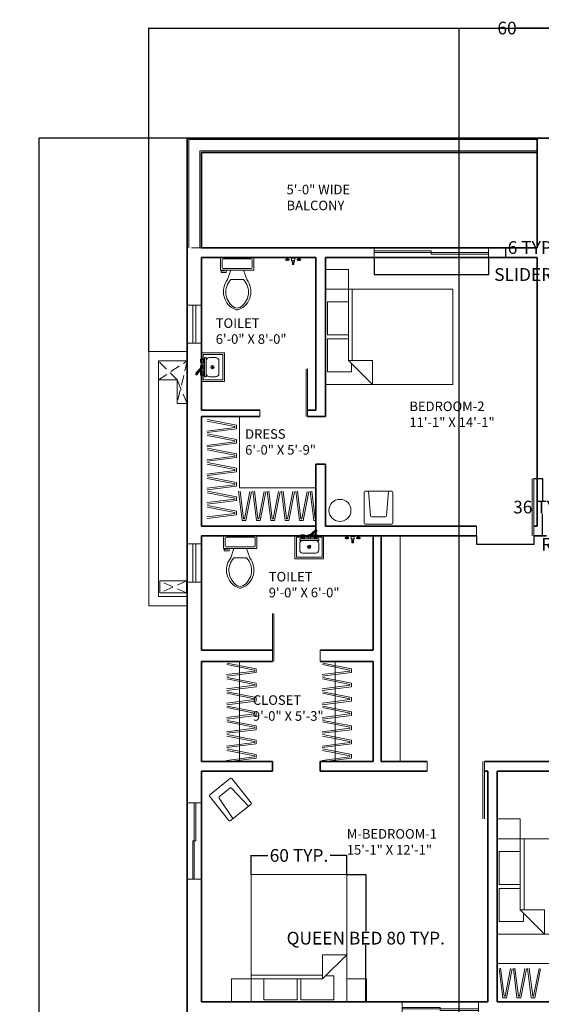
# Model space of a CAD drawing. Units: inches. Extents: x 3343 to 4790, y 1140 to 2641.
# Tile 3 of 10: x 3343 to 3671, y 2022 to 2641. Entities that reach past the tile are written whole.
import ezdxf

# ---------------------------------------------------------------- set-up
doc = ezdxf.new("R2010")
doc.units = ezdxf.units.IN
doc.header["$LTSCALE"] = 5
doc.header["$MEASUREMENT"] = 0
doc.linetypes.add('HIDDEN', pattern=[0.375, 0.25, -0.125])
for name, color, linetype, lineweight in [('A-ANNO-DIMS', 2, 'Continuous', 18), ('A-AREA-IDEN', 7, 'Continuous', 18), ('A-DOOR', 3, 'Continuous', 18), ('A-FLOR-CASE', 9, 'Continuous', 18), ('A-FLOR-FIXT', 9, 'Continuous', 18), ('A-FLOR-HIDN', 8, 'HIDDEN', 13), ('A-FLOR-RAIL', 7, 'Continuous', 18), ('A-FLOR-SHFT', 8, 'Continuous', 18), ('A-FURN', 8, 'Continuous', 13), ('A-GLAZ', 4, 'Continuous', 18), ('A-WALL', 7, 'Continuous', 35)]:
    doc.layers.add(name, color=color, linetype=linetype, lineweight=lineweight)
doc.styles.get("Standard").update_dxf_attribs({"font": 'arial.ttf'})
doc.dimstyles.get("Standard").update_dxf_attribs({"dimtxt": 8, "dimasz": 0.18, "dimexe": 0.18, "dimexo": 0.0625, "dimgap": 0.09, "dimtad": 0, "dimtih": 1, "dimtoh": 1, "dimdec": 1, "dimzin": 0, "dimdsep": 46, "dimlunit": 3, "dimtxsty": 'Standard', "dimcen": 0.09, "dimadec": 0, "dimazin": 0, "dimtfac": 1, "dimtdec": 1, "dimtofl": 0, "dimtmove": 0, "dimatfit": 3, "dimfxl": 1, "dimtolj": 1, "dimtzin": 0, "dimarcsym": 0})

# ---------------------------------------------------------------- blocks, each defined once
blk = doc.blocks.new('Bed - Queen')
for p, q in [((0, -80.00003), (0, 0)), ((0, 0), (59.99999, 0)), ((59.99999, 0), (59.99999, -80.00003)), ((7.99999, -1.2), (28.79998, -1.2)), ((7.99999, -14.4), (7.99999, -1.2)), ((28.79998, -1.2), (28.79998, -14.4)), ((31.19999, -1.2), (51.99999, -1.2)), ((31.19999, -14.4), (31.19999, -1.2)), ((51.99999, -1.2), (51.99999, -16.4)), ((0, -14.4), (44.8, -14.4)), ((44.8, -16.8), (0, -16.8)), ((59.99999, -29.6), (44.8, -14.4)), ((44.8, -14.4), (44.8, -29.6)), ((51.99999, -16.4), (46.79936, -16.4)), ((44.8, -29.6), (59.99999, -29.6)), ((59.99999, -80.00003), (0, -80.00003))]:
    blk.add_line(p, q)
blk = doc.blocks.new('Toilet - top')
for p, q in [((9.5, -6), (9.5, -2)), ((-10, -8.5), (-8, -8.5)), ((-10, -9.5), (-10, -8.5)), ((-7, -9.5), (-10, -9.5)), ((-8, -8.5), (-8, -8)), ((-7, -8), (-7, -9.5)), ((-4, -8), (-6, -14)), ((4, -8), (6, -14)), ((4, -14), (-4, -14))]:
    blk.add_line(p, q)
blk.add_lwpolyline([(10.5, -8), (10.5, 0), (-10.5, 0), (-10.5, -8)], close=True)
for points in [[(-9.5, -2), (-9.5, -6)], [(8.5, -1), (-8.5, -1)], [(-8.5, -7), (8.5, -7)]]:
    blk.add_lwpolyline(points)
for centre, radius, start, end in [((-8.62, -1.88), 0.884, 81.8699, 188.1301), ((-8.62, -6.12), 0.884, 171.8699, 278.1301), ((8.62, -1.88), 0.884, 351.8699, 98.1301), ((8.62, -6.12), 0.884, 261.8699, 8.1301), ((3.52, -21.58), 12.17, 141.46911, 247.97143), ((4.2, -21.82), 11.33, 136.36773, 238.94682), ((-3.52, -21.58), 12.17, 292.02843, 38.53071), ((-4.2, -21.82), 11.33, 301.05301, 43.63209), ((0, -27.88), 4, 245.73182, 294.26817), ((0, -29), 4, 254.86053, 285.13947)]:
    blk.add_arc(centre, radius, start, end)
blk = doc.blocks.new('Faucet - kit sink front')
for p, q in [((-0.25, 3), (3.75, 6.5)), ((3.75, 6), (3.75, 6.5)), ((3.75, 6.5), (4.75, 6.5)), ((4.75, 6.5), (4.75, 6)), ((-4.5, 1), (-4.5, 1.5)), ((-3.5, 1.5), (-3.5, 1)), ((-0.75, 3.5), (0.3192, 3.5)), ((-0.75, 1), (-0.75, 3.5)), ((3.75, 6), (-0.25, 2.5)), ((-0.25, 2.5), (-0.25, 3)), ((0.75, 2.5), (-0.25, 2.5)), ((4.1921, 5.5041), (0.75, 2.5)), ((0.75, 2.5), (0.75, 1)), ((3.5, 1.5), (3.5, 1)), ((3.75, 5.5), (3.75, 6)), ((4.75, 6), (3.75, 6)), ((4.75, 5.5), (3.75, 5.5)), ((4.5, 1), (4.5, 1.5)), ((4.75, 6), (4.75, 5.5))]:
    blk.add_line(p, q)
for points in [[(-6, 0), (-6, 1), (6, 1), (6, 0)], [(-5.5, 2.5), (-5.5, 3.25), (-4.5, 3.25), (-4.5, 2.5)], [(5.5, 2.5), (5.5, 3.25), (4.5, 3.25), (4.5, 2.5)]]:
    blk.add_lwpolyline(points, close=True)
for points in [[(-5, 3.2513), (-5, 3.5), (-3, 3.5), (-3, 1.5), (-5, 1.5), (-5, 2.5)], [(5, 3.2513), (5, 3.5), (3, 3.5), (3, 1.5), (5, 1.5), (5, 2.5)]]:
    blk.add_lwpolyline(points)
blk = doc.blocks.new('Faucet - Bathroom front')
for p, q in [((-5, 0), (-2.25, 0)), ((-4.5087, 0.25), (-2.7408, 0.25)), ((-4, 1.625), (-4.25, 1.625)), ((-4, 1.375), (-4.25, 1.375)), ((-3.1442, 0.75), (-4.0979, 0.75)), ((-3.25, 1.625), (-3, 1.625)), ((-3.25, 1.375), (-3, 1.375)), ((-1.5, 0), (1.5, 0)), ((-1, 0.5), (1, 0.5)), ((-0.5, 4.25), (0.5, 4.25)), ((0.5, 3.75), (-0.5, 3.75)), ((-0.5, 3), (0.5, 3)), ((0.5, 2), (-0.5, 2)), ((-0.25, 3), (-0.25, 3.5)), ((0.25, 3.5), (0.25, 3)), ((2.25, 0), (5, 0)), ((2.7413, 0.25), (4.5092, 0.25)), ((3.25, 1.625), (3, 1.625)), ((3.25, 1.375), (3, 1.375)), ((4.1058, 0.75), (3.1521, 0.75)), ((4, 1.625), (4.25, 1.625)), ((4, 1.375), (4.25, 1.375))]:
    blk.add_line(p, q)
for points in [[(-4, 1), (-4, 2), (-3.25, 2), (-3.25, 1)], [(3.25, 1), (3.25, 2), (4, 2), (4, 1)]]:
    blk.add_lwpolyline(points, close=True)
for points in [[(-0.5, 3.75), (-0.5, 4.25)], [(-0.25, 4.5), (0.25, 4.5)], [(0.25, 3.5), (-0.25, 3.5)], [(0.5, 4.25), (0.5, 3.75)]]:
    blk.add_lwpolyline(points)
for centre in [(-4.5, 1.5), (-3.625, 1.5), (-2.75, 1.5), (2.75, 1.5), (3.625, 1.5), (4.5, 1.5)]:
    blk.add_circle(centre, 0.2795)
for centre, radius, start, end in [((-5.375, 1.375), 1.4252, 285.2551, 344.7449), ((-1.875, 1.375), 1.4252, 195.2551, 254.7449), ((-0.7962, -0.2038), 0.7327, 106.1502, 163.8498), ((3, 1), 4.0311, 150.2551, 187.125), ((0.6413, 2.5), 1.246, 156.3417, 203.6583), ((-0.2575, 4.2575), 0.2426, 88.22243, 181.7776), ((-0.2575, 3.7425), 0.2426, 178.2224, 271.7776), ((0.2575, 4.2575), 0.2426, 358.2224, 91.77757), ((0.2575, 3.7425), 0.2426, 268.2224, 1.777565), ((-3, 1), 4.0311, 352.875, 29.74488), ((-0.6413, 2.5), 1.246, 336.3417, 23.65835), ((0.7962, -0.2038), 0.7327, 16.1502, 73.84979), ((1.875, 1.375), 1.4252, 285.2551, 344.7449), ((5.375, 1.375), 1.4252, 195.2551, 254.7449)]:
    blk.add_arc(centre, radius, start, end)
blk = doc.blocks.new('CHAIR-SIDE')
for p, q in [((0, 0.6), (0, 20.1)), ((0.6, 20.7), (17.39, 20.7)), ((2.68, 20.7), (3.95, 5.17)), ((15.31, 20.7), (14.03, 5.17)), ((17.98, 20.1), (17.98, 0.6)), ((17.39, 0), (0.6, 0)), ((13.44, 4.62), (4.54, 4.62))]:
    blk.add_line(p, q)
for centre, start, end in [((0.6, 20.1), 90, 180), ((17.39, 20.1), 0, 90), ((0.6, 0.6), 180, 270), ((4.54, 5.22), 184.67931, 270), ((13.44, 5.22), 270, 355.32069), ((17.39, 0.6), 270, 0)]:
    blk.add_arc(centre, 0.595, start, end)
blk = doc.blocks.new('SINK-BOWL-WITH-DRAIN')
for p, q in [((8.58, 9.03), (6.47, 9.03)), ((7.52, 10.09), (7.52, 7.97))]:
    blk.add_line(p, q)
for points in [[(14.44, 0), (0, 0), (0, 18.06), (14.44, 18.06)], [(1, 1), (1, 17.06), (13.44, 17.06), (13.44, 1)]]:
    blk.add_lwpolyline(points, close=True)
blk.add_lwpolyline([(9.44, 15.06), (5.44, 15.06, 0.414214), (3.44, 13.06), (3.44, 5, 0.414214), (5.44, 3), (9.44, 3, 0.414214), (11.44, 5), (11.44, 13.06, 0.414214)], format="xyb", close=True)
blk.add_circle((7.52, 9.03), 1.06)
blk = doc.blocks.new('WINDOW-48IN-SLIDING-JAMB9')
for p, q in [((0, 9), (0, 0)), ((48, 9), (48, 0)), ((0, 5.5), (24, 5.5)), ((0, 4.5), (48, 4.5)), ((24, 5.5), (24, 3.5)), ((24, 3.5), (48, 3.5))]:
    blk.add_line(p, q)
blk = doc.blocks.new('WINDOW-24IN-FIXED')
for p, q in [((0, 9), (0, 0)), ((24, 9), (24, 0)), ((0, 5.5), (24, 5.5)), ((0, 3.5), (24, 3.5))]:
    blk.add_line(p, q)
blk = doc.blocks.new('WINDOW-72IN-SLIDING')
at = {"ltscale": 5}
for p, q in [((0, 6), (0, 0)), ((0, 4), (36, 4)), ((0, 3), (72, 3)), ((36, 4), (36, 2)), ((36, 2), (72, 2)), ((72, 6), (72, 0))]:
    blk.add_line(p, q, dxfattribs=at)
blk = doc.blocks.new('DOOR-36IN-6IN-JAMB-DBL-LINE')
at = {"ltscale": 5}
for p, q in [((35, 0), (35, 36)), ((36, 0), (36, 36)), ((0, 6), (0, 0)), ((36, 6), (36, 0))]:
    blk.add_line(p, q, dxfattribs=at)
blk = doc.blocks.new('DOOR-30IN-4IN-JAMB-DBL-LINE')
at = {"ltscale": 5}
for p, q in [((29, 0), (29, 30)), ((30, 0), (30, 30)), ((0, 4), (0, 0)), ((30, 4), (30, 0))]:
    blk.add_line(p, q, dxfattribs=at)
blk = doc.blocks.new('WARDROBE-HANGER')
for points in [[(0.22, 7.19), (17.51, 3.78), (17.51, 3.18), (0, 0.99)], [(0.41, 8.17), (18.51, 4.61), (18.51, 2.3), (0.12, 0)]]:
    blk.add_lwpolyline(points)
blk = doc.blocks.new('NIGHTSTAND')
blk.add_lwpolyline([(12.43, 0), (0, 0), (0, 14.43), (12.43, 14.43)], close=True)
blk = doc.blocks.new('*D43')
at = {"layer": 'A-ANNO-DIMS', "color": 0, "lineweight": -2, "ltscale": 5, "transparency": 16777216}
for p, q in [((3548.51, 2103.16), (3560.63, 2103.16)), ((3560.45, 2102.98), (3560.45, 2067.63)), ((3560.45, 2023.34), (3560.45, 2058.69)), ((3548.51, 2023.16), (3560.63, 2023.16))]:
    blk.add_line(p, q, dxfattribs=at)
at = {"layer": 'A-ANNO-DIMS', "color": 0, "ltscale": 5, "transparency": 16777216}
for points in [[(3560.42, 2102.98), (3560.48, 2102.98), (3560.45, 2103.16)], [(3560.42, 2023.34), (3560.48, 2023.34), (3560.45, 2023.16)]]:
    blk.add_solid(points, dxfattribs=at)
at = {"layer": 'Defpoints', "color": 0, "ltscale": 5, "transparency": 16777216}
for p in [(3548.45, 2103.16), (3548.45, 2023.16), (3560.45, 2023.16)]:
    blk.add_point(p, dxfattribs=at)
at = {"layer": 'A-ANNO-DIMS', "color": 0, "ltscale": 5, "transparency": 16777216, "insert": (3560.45, 2063.16), "char_height": 8, "attachment_point": 5}
blk.add_mtext('\\A1;QUEEN BED 80 TYP.', dxfattribs=at)
blk = doc.blocks.new('*D44')
at = {"layer": 'A-ANNO-DIMS', "color": 0, "lineweight": -2, "ltscale": 5, "transparency": 16777216}
for p, q in [((3488.45, 2103.22), (3488.45, 2115.34)), ((3488.63, 2115.16), (3498.86, 2115.16)), ((3548.27, 2115.16), (3538.03, 2115.16)), ((3548.45, 2103.22), (3548.45, 2115.34))]:
    blk.add_line(p, q, dxfattribs=at)
at = {"layer": 'A-ANNO-DIMS', "color": 0, "ltscale": 5, "transparency": 16777216}
for points in [[(3488.63, 2115.19), (3488.63, 2115.13), (3488.45, 2115.16)], [(3548.27, 2115.19), (3548.27, 2115.13), (3548.45, 2115.16)]]:
    blk.add_solid(points, dxfattribs=at)
at = {"layer": 'Defpoints', "color": 0, "ltscale": 5, "transparency": 16777216}
for p in [(3548.45, 2115.16), (3488.45, 2103.16), (3548.45, 2103.16)]:
    blk.add_point(p, dxfattribs=at)
at = {"layer": 'A-ANNO-DIMS', "color": 0, "ltscale": 5, "transparency": 16777216, "insert": (3518.45, 2115.16), "char_height": 8, "attachment_point": 5}
blk.add_mtext('\\A1;60 TYP.', dxfattribs=at)
blk = doc.blocks.new('*D61')
at = {"layer": 'A-ANNO-DIMS', "color": 0, "lineweight": -2, "ltscale": 5, "transparency": 16777216}
for p, q in [((3565.63, 2491.1), (3565.63, 2480.18)), ((3637.63, 2491.1), (3637.63, 2480.18)), ((3565.81, 2480.36), (3637.45, 2480.36)), ((3637.63, 2480.36), (3637.81, 2480.36))]:
    blk.add_line(p, q, dxfattribs=at)
at = {"layer": 'A-ANNO-DIMS', "color": 0, "ltscale": 5, "transparency": 16777216}
for points in [[(3565.81, 2480.39), (3565.81, 2480.33), (3565.63, 2480.36)], [(3637.45, 2480.39), (3637.45, 2480.33), (3637.63, 2480.36)]]:
    blk.add_solid(points, dxfattribs=at)
at = {"layer": 'Defpoints', "color": 0, "ltscale": 5, "transparency": 16777216}
for p in [(3565.63, 2491.16), (3637.63, 2491.16), (3637.63, 2480.36)]:
    blk.add_point(p, dxfattribs=at)
at = {"layer": 'A-ANNO-DIMS', "color": 0, "ltscale": 5, "transparency": 16777216, "insert": (3679.09, 2480.36), "char_height": 8, "attachment_point": 5}
blk.add_mtext('\\A1;SLIDER 72 TYP.', dxfattribs=at)
blk = doc.blocks.new('*D62')
at = {"layer": 'A-ANNO-DIMS', "color": 0, "lineweight": -2, "ltscale": 5, "transparency": 16777216}
for p, q in [((3637.69, 2497.16), (3648.61, 2497.16)), ((3648.43, 2497.16), (3648.43, 2497.34)), ((3648.43, 2497.34), (3648.61, 2497.34)), ((3648.43, 2491.34), (3648.43, 2496.98)), ((3637.69, 2491.16), (3648.61, 2491.16))]:
    blk.add_line(p, q, dxfattribs=at)
at = {"layer": 'A-ANNO-DIMS', "color": 0, "ltscale": 5, "transparency": 16777216}
for points in [[(3648.4, 2496.98), (3648.46, 2496.98), (3648.43, 2497.16)], [(3648.4, 2491.34), (3648.46, 2491.34), (3648.43, 2491.16)]]:
    blk.add_solid(points, dxfattribs=at)
at = {"layer": 'Defpoints', "color": 0, "ltscale": 5, "transparency": 16777216}
for p in [(3637.63, 2497.16), (3648.43, 2497.16), (3637.63, 2491.16)]:
    blk.add_point(p, dxfattribs=at)
at = {"layer": 'A-ANNO-DIMS', "color": 0, "ltscale": 5, "transparency": 16777216, "insert": (3665.08, 2497.34), "char_height": 8, "attachment_point": 5}
blk.add_mtext('\\A1;6 TYP.', dxfattribs=at)
blk = doc.blocks.new('*D65')
at = {"layer": 'A-ANNO-DIMS', "color": 0, "lineweight": -2, "ltscale": 5, "transparency": 16777216}
for p, q in [((3630.13, 2316.1), (3630.13, 2310.58)), ((3666.13, 2316.1), (3666.13, 2310.58)), ((3630.31, 2310.76), (3665.95, 2310.76)), ((3666.13, 2310.76), (3666.31, 2310.76))]:
    blk.add_line(p, q, dxfattribs=at)
at = {"layer": 'A-ANNO-DIMS', "color": 0, "ltscale": 5, "transparency": 16777216}
for points in [[(3630.31, 2310.79), (3630.31, 2310.73), (3630.13, 2310.76)], [(3665.95, 2310.79), (3665.95, 2310.73), (3666.13, 2310.76)]]:
    blk.add_solid(points, dxfattribs=at)
at = {"layer": 'Defpoints', "color": 0, "ltscale": 5, "transparency": 16777216}
for p in [(3630.13, 2316.16), (3666.13, 2316.16), (3666.13, 2310.76)]:
    blk.add_point(p, dxfattribs=at)
at = {"layer": 'A-ANNO-DIMS', "color": 0, "ltscale": 5, "transparency": 16777216, "insert": (3722.92, 2310.76), "char_height": 8, "attachment_point": 5}
blk.add_mtext('\\A1;ROOM DOOR 36 TYP.', dxfattribs=at)
blk = doc.blocks.new('*D66')
at = {"layer": 'A-ANNO-DIMS', "color": 0, "lineweight": -2, "ltscale": 5, "transparency": 16777216}
for p, q in [((3666.19, 2352.16), (3671.71, 2352.16)), ((3671.53, 2351.98), (3671.53, 2338.34)), ((3671.53, 2316.34), (3671.53, 2329.98)), ((3666.19, 2316.16), (3671.71, 2316.16))]:
    blk.add_line(p, q, dxfattribs=at)
at = {"layer": 'A-ANNO-DIMS', "color": 0, "ltscale": 5, "transparency": 16777216}
for points in [[(3671.5, 2351.98), (3671.56, 2351.98), (3671.53, 2352.16)], [(3671.5, 2316.34), (3671.56, 2316.34), (3671.53, 2316.16)]]:
    blk.add_solid(points, dxfattribs=at)
at = {"layer": 'Defpoints', "color": 0, "ltscale": 5, "transparency": 16777216}
for p in [(3666.13, 2352.16), (3671.53, 2352.16), (3666.13, 2316.16)]:
    blk.add_point(p, dxfattribs=at)
at = {"layer": 'A-ANNO-DIMS', "color": 0, "ltscale": 5, "transparency": 16777216, "insert": (3671.53, 2334.16), "char_height": 8, "attachment_point": 5}
blk.add_mtext('\\A1;36 TYP.', dxfattribs=at)
blk = doc.blocks.new('*D83')
at = {"layer": 'A-ANNO-DIMS', "color": 0, "lineweight": -2, "ltscale": 5, "transparency": 16777216}
for p, q in [((3424.13, 2432.05), (3424.13, 2635.49)), ((3424.31, 2635.31), (4052.48, 2635.31)), ((4703.95, 2635.31), (4075.77, 2635.31)), ((4704.13, 2197.22), (4704.13, 2635.49))]:
    blk.add_line(p, q, dxfattribs=at)
at = {"layer": 'A-ANNO-DIMS', "color": 0, "ltscale": 5, "transparency": 16777216}
for points in [[(3424.31, 2635.34), (3424.31, 2635.28), (3424.13, 2635.31)], [(4703.95, 2635.34), (4703.95, 2635.28), (4704.13, 2635.31)]]:
    blk.add_solid(points, dxfattribs=at)
at = {"layer": 'Defpoints', "color": 0, "ltscale": 5, "transparency": 16777216}
for p in [(4704.13, 2635.31), (3424.13, 2431.99), (4704.13, 2197.16)]:
    blk.add_point(p, dxfattribs=at)
at = {"layer": 'A-ANNO-DIMS', "color": 0, "ltscale": 5, "transparency": 16777216, "insert": (4064.13, 2635.31), "char_height": 8, "attachment_point": 5}
blk.add_mtext('\\A1;1280', dxfattribs=at)
blk = doc.blocks.new('*D84')
at = {"layer": 'A-ANNO-DIMS', "color": 0, "lineweight": -2, "ltscale": 5, "transparency": 16777216}
for p, q in [((3448.07, 2566.16), (3354.8, 2566.16)), ((3354.98, 2565.98), (3354.98, 1894.31)), ((3354.98, 1214.29), (3354.98, 1885.96)), ((4015.58, 1214.11), (3354.8, 1214.11))]:
    blk.add_line(p, q, dxfattribs=at)
at = {"layer": 'A-ANNO-DIMS', "color": 0, "ltscale": 5, "transparency": 16777216}
for points in [[(3354.95, 2565.98), (3355.01, 2565.98), (3354.98, 2566.16)], [(3354.95, 1214.29), (3355.01, 1214.29), (3354.98, 1214.11)]]:
    blk.add_solid(points, dxfattribs=at)
at = {"layer": 'Defpoints', "color": 0, "ltscale": 5, "transparency": 16777216}
for p in [(3448.13, 2566.16), (3354.98, 1214.11), (4015.65, 1214.11)]:
    blk.add_point(p, dxfattribs=at)
at = {"layer": 'A-ANNO-DIMS', "color": 0, "ltscale": 5, "transparency": 16777216, "insert": (3354.98, 1890.14), "char_height": 8, "attachment_point": 5}
blk.add_mtext('\\A1;1352', dxfattribs=at)
blk = doc.blocks.new('*D96')
at = {"layer": 'A-ANNO-DIMS', "color": 0, "lineweight": -2, "ltscale": 5, "transparency": 16777216}
for p, q in [((3619.25, 1835.73), (3619.25, 2635.49)), ((3619.43, 2635.31), (3643.42, 2635.31)), ((3679.07, 2635.31), (3655.08, 2635.31)), ((3679.25, 1835.73), (3679.25, 2635.49))]:
    blk.add_line(p, q, dxfattribs=at)
at = {"layer": 'A-ANNO-DIMS', "color": 0, "ltscale": 5, "transparency": 16777216}
for points in [[(3619.43, 2635.34), (3619.43, 2635.28), (3619.25, 2635.31)], [(3679.07, 2635.34), (3679.07, 2635.28), (3679.25, 2635.31)]]:
    blk.add_solid(points, dxfattribs=at)
at = {"layer": 'Defpoints', "color": 0, "ltscale": 5, "transparency": 16777216}
for p in [(3679.25, 2635.31), (3619.25, 1835.67), (3679.25, 1835.67)]:
    blk.add_point(p, dxfattribs=at)
at = {"layer": 'A-ANNO-DIMS', "color": 0, "ltscale": 5, "transparency": 16777216, "insert": (3649.25, 2635.31), "char_height": 8, "attachment_point": 5}
blk.add_mtext('\\A1;60', dxfattribs=at)

msp = doc.modelspace()

# ---------------------------------------------------------------- linework, layer by layer
at = {"layer": 'A-DOOR', "ltscale": 5}
for p, q in [((3501.726, 2237.161), (3501.726, 2267.161)), ((3502.726, 2237.161), (3502.726, 2267.161)), ((3501.726, 2237.161), (3501.726, 2244.161)), ((3531.726, 2237.161), (3531.726, 2244.161))]:
    msp.add_line(p, q, dxfattribs=at)
at = {"layer": 'A-FLOR-CASE'}
for p, q in [((3481.13, 2391.161), (3481.13, 2346.161)), ((3481.13, 2237.161), (3481.13, 2174.161)), ((3541.13, 2237.161), (3541.13, 2174.161))]:
    msp.add_line(p, q, dxfattribs=at)
at = {"layer": 'A-FLOR-CASE', "ltscale": 5}
for p, q in [((3529.13, 2346.161), (3481.13, 2346.161)), ((3582.13, 2316.161), (3582.13, 2174.161)), ((3775.13, 2047.161), (3643.13, 2047.161))]:
    msp.add_line(p, q, dxfattribs=at)
at = {"layer": 'A-FLOR-CASE'}
for points in [[(3529.13, 2325.721), (3527.768, 2325.721), (3525.471, 2344.112)], [(3529.13, 2326.721), (3528.651, 2326.721), (3526.464, 2344.236)]]:
    msp.add_lwpolyline(points, dxfattribs=at)
at = {"layer": 'A-FLOR-HIDN', "ltscale": 5}
for p, q in [((3457.13, 2497.161), (3448.13, 2497.161)), ((3430.13, 2414.14), (3448.13, 2425.992)), ((3441.822, 2414.14), (3430.13, 2425.992)), ((3448.13, 2425.992), (3441.822, 2399.342)), ((3448.13, 2399.342), (3441.822, 2414.14)), ((3447.792, 2280.206), (3431.001, 2287.69)), ((3447.792, 2287.69), (3431.001, 2280.206))]:
    msp.add_line(p, q, dxfattribs=at)
at = {"layer": 'A-FLOR-RAIL', "ltscale": 5}
for p, q in [((3668.13, 2565.161), (3449.13, 2565.161)), ((3668.13, 2558.161), (3456.13, 2558.161))]:
    msp.add_line(p, q, dxfattribs=at)
at = {"layer": 'A-FLOR-RAIL'}
for p, q in [((3449.13, 2565.161), (3449.13, 2497.161)), ((3456.13, 2558.161), (3456.13, 2497.161))]:
    msp.add_line(p, q, dxfattribs=at)
at = {"layer": 'A-FLOR-SHFT', "ltscale": 5}
for p, q in [((3430.13, 2414.14), (3441.822, 2414.14)), ((3441.822, 2414.14), (3441.822, 2399.342)), ((3441.822, 2399.342), (3448.13, 2399.342))]:
    msp.add_line(p, q, dxfattribs=at)
for points in [[(3448.13, 2431.992), (3424.13, 2431.992), (3424.13, 2271.97), (3448.13, 2271.97)], [(3448.13, 2425.992), (3430.13, 2425.992), (3430.13, 2277.97), (3448.13, 2277.97)]]:
    msp.add_lwpolyline(points, dxfattribs=at)
msp.add_lwpolyline([(3431.001, 2280.206), (3447.792, 2280.206), (3447.792, 2287.69), (3431.001, 2287.69)], close=True, dxfattribs=at)
at = {"layer": 'A-FURN'}
msp.add_circle((3544.194, 2332.038), 6.927, dxfattribs=at)
at = {"layer": 'A-WALL', "ltscale": 5}
for p, q in [((3977.13, 2566.161), (3448.13, 2566.161)), ((3668.13, 2557.161), (3457.13, 2557.161)), ((3668.13, 2497.161), (3457.13, 2497.161)), ((3529.13, 2491.161), (3457.13, 2491.161)), ((3668.13, 2491.161), (3535.13, 2491.161)), ((3493.908, 2395.161), (3457.13, 2395.161)), ((3493.908, 2391.161), (3457.13, 2391.161)), ((3529.13, 2395.161), (3523.908, 2395.161)), ((3529.13, 2391.161), (3523.908, 2391.161)), ((3529.13, 2391.161), (3535.13, 2391.161)), ((3529.13, 2361.161), (3535.13, 2361.161)), ((3529.13, 2322.161), (3457.13, 2322.161)), ((3529.13, 2322.161), (3529.13, 2316.161)), ((3630.13, 2322.161), (3535.13, 2322.161)), ((3668.13, 2322.161), (3666.13, 2322.161)), ((3565.13, 2316.161), (3457.13, 2316.161)), ((3565.13, 2316.161), (3570.13, 2316.161)), ((3570.13, 2316.161), (3570.13, 2174.161)), ((3630.13, 2316.161), (3570.13, 2316.161)), ((3674.13, 2316.161), (3666.13, 2316.161)), ((3501.726, 2244.161), (3457.13, 2244.161)), ((3565.13, 2244.161), (3531.726, 2244.161)), ((3501.726, 2237.161), (3457.13, 2237.161)), ((3565.13, 2237.161), (3531.726, 2237.161)), ((3501.726, 2174.161), (3457.13, 2174.161)), ((3501.726, 2174.161), (3501.726, 2168.161)), ((3565.13, 2174.161), (3531.726, 2174.161)), ((3531.726, 2174.161), (3531.726, 2168.161)), ((3599.13, 2174.161), (3570.13, 2174.161)), ((3737.13, 2174.161), (3635.13, 2174.161)), ((3501.726, 2168.161), (3457.13, 2168.161)), ((3599.13, 2168.161), (3531.726, 2168.161)), ((3637.13, 2168.161), (3635.13, 2168.161)), ((3737.13, 2168.161), (3643.13, 2168.161)), ((3637.13, 2023.161), (3457.13, 2023.161)), ((3775.13, 2023.161), (3643.13, 2023.161))]:
    msp.add_line(p, q, dxfattribs=at)
at = {"layer": 'A-WALL'}
for p, q in [((3448.13, 2566.161), (3448.13, 2014.161)), ((3668.13, 2566.161), (3668.13, 2497.161)), ((3457.13, 2557.161), (3457.13, 2497.161)), ((3457.13, 2491.161), (3457.13, 2395.161)), ((3529.13, 2491.161), (3529.13, 2395.161)), ((3535.13, 2491.161), (3535.13, 2391.161)), ((3668.13, 2491.161), (3668.13, 2322.161)), ((3457.13, 2391.161), (3457.13, 2322.161)), ((3529.13, 2361.161), (3529.13, 2322.161)), ((3535.13, 2361.161), (3535.13, 2322.161)), ((3457.13, 2316.161), (3457.13, 2244.161)), ((3565.13, 2316.161), (3565.13, 2244.161)), ((3457.13, 2237.161), (3457.13, 2174.161)), ((3565.13, 2237.161), (3565.13, 2174.161)), ((3457.13, 2168.161), (3457.13, 2023.161)), ((3637.13, 2168.161), (3637.13, 2023.161)), ((3643.13, 2168.161), (3643.13, 2023.161))]:
    msp.add_line(p, q, dxfattribs=at)

# ---------------------------------------------------------------- block references
at = {"layer": 'A-DOOR'}
for name, p in [('DOOR-30IN-4IN-JAMB-DBL-LINE', (3493.908, 2391.161)), ('DOOR-36IN-6IN-JAMB-DBL-LINE', (3630.13, 2316.161))]:
    msp.add_blockref(name, p, dxfattribs=at)
at = {"layer": 'A-DOOR', "extrusion": (0, 0, -1), "zscale": -1, "rotation": 180}
msp.add_blockref('DOOR-36IN-6IN-JAMB-DBL-LINE', (-3599.13, 2174.161), dxfattribs=at)
at = {"layer": 'A-FLOR-CASE'}
for p in [(3460.605, 2380.957), (3460.605, 2371.957), (3460.605, 2362.957), (3460.605, 2353.957), (3460.605, 2344.957), (3460.605, 2335.957), (3460.605, 2326.957), (3472.963, 2227.918), (3532.963, 2227.918), (3472.963, 2218.918), (3532.963, 2218.918), (3472.963, 2209.918), (3532.963, 2209.918), (3472.963, 2200.918), (3532.963, 2200.918), (3472.963, 2191.918), (3532.963, 2191.918), (3472.963, 2182.918), (3532.963, 2182.918), (3472.963, 2173.918), (3532.963, 2173.918)]:
    msp.add_blockref('WARDROBE-HANGER', p, dxfattribs=at)
for p, rotation in [((3480.471, 2344.236), 270.000000000001), ((3489.471, 2344.236), 270.000000000006), ((3498.471, 2344.236), 270.000000000001), ((3507.471, 2344.236), 270.000000000006), ((3516.471, 2344.236), 269.9999999999961), ((3644.227, 2044.218), 270.000000000011), ((3653.227, 2044.218), 270.0000000000061), ((3662.227, 2044.218), 270.000000000011)]:
    msp.add_blockref('WARDROBE-HANGER', p, dxfattribs=dict(at, rotation=rotation))
at = {"layer": 'A-FLOR-FIXT'}
for name, p in [('Toilet - top', (3479.592, 2491.161)), ('Toilet - top', (3481.511, 2316.161)), ('Faucet - kit sink front', (3524.928, 2313.161))]:
    msp.add_blockref(name, p, dxfattribs=at)
for name, p, rotation in [('Faucet - Bathroom front', (3514.785, 2491.161), 180), ('SINK-BOWL-WITH-DRAIN', (3533.959, 2301.724), 89.99999999999655), ('Faucet - Bathroom front', (3552.203, 2316.147), 180)]:
    msp.add_blockref(name, p, dxfattribs=dict(at, rotation=rotation))
at = {"layer": 'A-FLOR-FIXT', "xscale": -1, "rotation": 90}
msp.add_blockref('Faucet - kit sink front', (3460.13, 2422.135), dxfattribs=at)
at = {"layer": 'A-FLOR-FIXT', "extrusion": (0, 0, -1), "zscale": -1}
msp.add_blockref('SINK-BOWL-WITH-DRAIN', (-3471.566, 2413.104), dxfattribs=at)
at = {"layer": 'A-FURN'}
for name, p, rotation in [('NIGHTSTAND', (3535.13, 2483.589), 269.9999999999955), ('CHAIR-SIDE', (3475.94, 2164.005), 218.5043955807355), ('NIGHTSTAND', (3643.13, 2138.089), 269.9999999999983)]:
    msp.add_blockref(name, p, dxfattribs=dict(at, rotation=rotation))
at = {"layer": 'A-FURN', "xscale": -1}
for p, rotation in [((3535.13, 2471.161), 90), ((3643.13, 2125.661), 90), ((3488.447, 2023.161), 180)]:
    msp.add_blockref('Bed - Queen', p, dxfattribs=dict(at, rotation=rotation))
at = {"layer": 'A-FURN'}
for name, p in [('CHAIR-SIDE', (3559.514, 2323.407)), ('NIGHTSTAND', (3476.019, 2023.161)), ('NIGHTSTAND', (3548.447, 2023.161))]:
    msp.add_blockref(name, p, dxfattribs=at)
at = {"layer": 'A-GLAZ'}
for name, p in [('WINDOW-72IN-SLIDING', (3565.63, 2491.161)), ('WINDOW-48IN-SLIDING-JAMB9', (3583.248, 2014.161))]:
    msp.add_blockref(name, p, dxfattribs=at)
for name, p, rotation in [('WINDOW-24IN-FIXED', (3457.13, 2437.144), 89.9999999999986), ('WINDOW-24IN-FIXED', (3448.13, 2310.951), 270.0000000000005), ('WINDOW-48IN-SLIDING-JAMB9', (3457.13, 2100.255), 90.00000000000178)]:
    msp.add_blockref(name, p, dxfattribs=dict(at, rotation=rotation))

# ---------------------------------------------------------------- texts
at = {"layer": 'A-AREA-IDEN', "ltscale": 5, "char_height": 6, "attachment_point": 1}
for s, insert in [('5\'-0" WIDE \\PBALCONY', (3510.646, 2536.793)), ('TOILET\\P6\'-0" X 8\'-0"', (3466.116, 2452.797)), ('BEDROOM-2\\P11\'-1" X 14\'-1"', (3587.89, 2400.51)), ('DRESS\\P6\'-0" X 5\'-9"', (3484.626, 2383.113)), ('TOILET\\P9\'-0" X 6\'-0"', (3499.444, 2293.405)), ('CLOSET\\P9\'-0" X 5\'-3"', (3489.471, 2215.823)), ('M-BEDROOM-1\\P15\'-1" X 12\'-1"', (3548.523, 2131.696))]:
    msp.add_mtext_dynamic_manual_height_columns(s, width=189.69543, gutter_width=1, heights=[0], dxfattribs=dict(at, insert=insert))

# ---------------------------------------------------------------- dimensions: what is measured, and where the dimension line sits
at = {"layer": 'A-ANNO-DIMS', "ltscale": 5}
for base, p1, p2, picture, middle in [((4704.13, 2635.311), (3424.13, 2431.992), (4704.13, 2197.161), '*D83', (4064.13, 2635.311)), ((3679.248, 2635.311), (3619.248, 1835.669), (3679.248, 1835.669), '*D96', (3649.248, 2635.311))]:
    dim = msp.add_linear_dim(base=base, p1=p1, p2=p2, dimstyle='Standard', override={"dimdec": 0, "dimlfac": 1, "dimrnd": 0, "dimzin": 0, "dimdsep": 46, "dimlunit": 2}, dxfattribs=at)
    dim.commit()
    dim.dimension.update_dxf_attribs({"geometry": picture, "text_midpoint": middle})
dim = msp.add_linear_dim(base=(3354.98, 1214.112), p1=(3448.13, 2566.161), p2=(4015.647, 1214.112), angle=90, dimstyle='Standard', override={"dimdec": 0, "dimlfac": 1, "dimrnd": 0, "dimzin": 0, "dimdsep": 46, "dimlunit": 2}, dxfattribs=at)
dim.commit()
dim.dimension.update_dxf_attribs({"geometry": '*D84', "text_midpoint": (3354.98, 1890.137)})
for base, p1, p2, angle, text, picture, middle in [((3648.43, 2497.161), (3637.63, 2491.161), (3637.63, 2497.161), 90, '<> TYP.', '*D62', (3665.084, 2497.341)), ((3671.53, 2352.161), (3666.13, 2316.161), (3666.13, 2352.161), 90, '<> TYP.', '*D66', (3671.53, 2334.161)), ((3560.447, 2023.161), (3548.447, 2103.161), (3548.447, 2023.161), 270, 'QUEEN BED <> TYP.', '*D43', (3560.447, 2063.161))]:
    dim = msp.add_linear_dim(base=base, p1=p1, p2=p2, angle=angle, text=text, dimstyle='Standard', override={"dimdec": 0, "dimlfac": 1, "dimrnd": 0, "dimzin": 0, "dimdsep": 46, "dimlunit": 2}, dxfattribs=at)
    dim.commit()
    dim.dimension.update_dxf_attribs({"geometry": picture, "text_midpoint": middle})
for base, p1, p2, text, picture, middle in [((3637.63, 2480.361), (3565.63, 2491.161), (3637.63, 2491.161), 'SLIDER <> TYP.', '*D61', (3679.089, 2480.361)), ((3666.13, 2310.761), (3630.13, 2316.161), (3666.13, 2316.161), 'ROOM DOOR <> TYP.', '*D65', (3722.915, 2310.761)), ((3548.447, 2115.161), (3488.447, 2103.161), (3548.447, 2103.161), '<> TYP.', '*D44', (3518.447, 2115.161))]:
    dim = msp.add_linear_dim(base=base, p1=p1, p2=p2, text=text, dimstyle='Standard', override={"dimdec": 0, "dimlfac": 1, "dimrnd": 0, "dimzin": 0, "dimdsep": 46, "dimlunit": 2}, dxfattribs=at)
    dim.commit()
    dim.dimension.update_dxf_attribs({"geometry": picture, "text_midpoint": middle})

doc.saveas('drawing.dxf')
